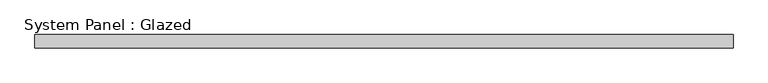
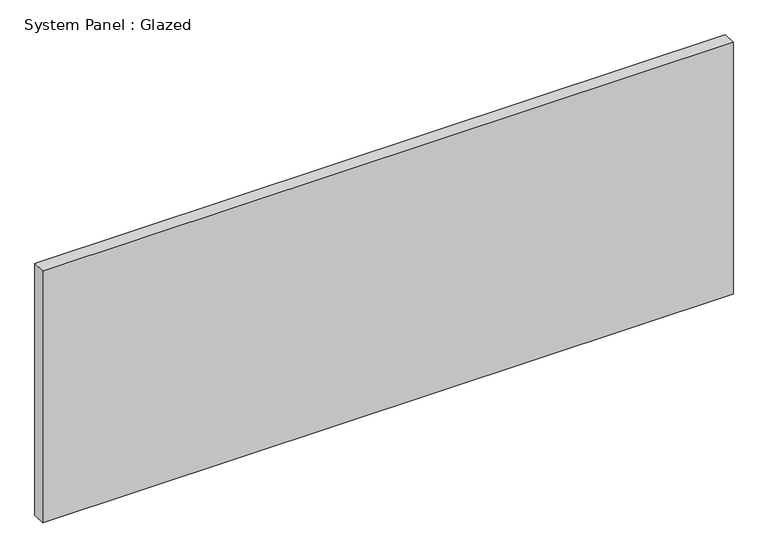
"""IFC4 building model written with IfcOpenShell, lengths in millimetres: plate geometry, System Panel : Glazed."""

from ifc_helpers import new_model, si_unit, origin, origin_with_axes, place, context, project, spatial, polyline, outline, extrude, source, transform, mapped, element, save


def system_panel_glazed_f09e76d7(model_context):
    return source(origin(), model_context, "Body", "SweptSolid", [
        extrude(outline(polyline([(666.7499999, -44.45), (-666.7499999, -44.45), (-666.7499999, -19.05), (666.7499999, -19.05), (666.7499999, -44.45)])), origin_with_axes(), (0.0, 0.0, 1.0), 514.35),
    ])


if __name__ == "__main__":
    model = new_model("IFC4")
    model_context = context("Model", 3, world=origin())
    ifc_project = project(units=[si_unit("LENGTHUNIT", "METRE", prefix="MILLI")], contexts=[model_context])
    site = spatial("IfcSite", under=ifc_project)
    building = spatial("IfcBuilding", under=site)
    placement = place(None, origin())
    system_panel_glazed_shape = system_panel_glazed_f09e76d7(model_context)
    element("IfcPlate", 1, ObjectType="System Panel : Glazed", at=placement, inside=building, context=model_context, shape_type="MappedRepresentation", body=[
        mapped(system_panel_glazed_shape, transform((0.0, 0.0, 0.0), x_axis=(1.0, 0.0, 0.0), y_axis=(0.0, 1.0, 0.0), z_axis=(0.0, 0.0, 1.0))),
    ])
    save(model, "model.ifc")

# Revit data of these elements
# Type "System Panel : Glazed"
#   Construction Type Id = "GSP4R"
#   Analytic Construction = "1/8 in Pilkington single glazing"
#   Visual Light Transmittance = 0.9
#   Solar Heat Gain Coefficient = 0.86
#   Heat Transfer Coefficient (U) = 1.18115 BTU/(h·ft²·°F)
#   Define Thermal Properties by = 1
# Element 1 (IfcPlate, "System Panel : Glazed")
#   Materials on its faces: "glass panel 223"
# Materials
#   "glass panel 223": class "Generic", colour RGB 120 120 120, transparency 0, Cost = 0
